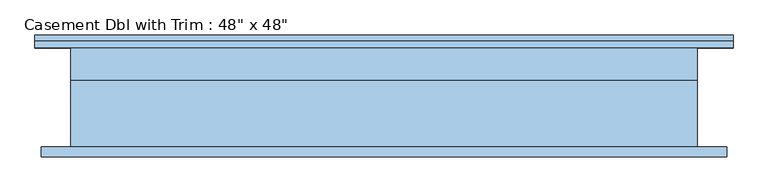
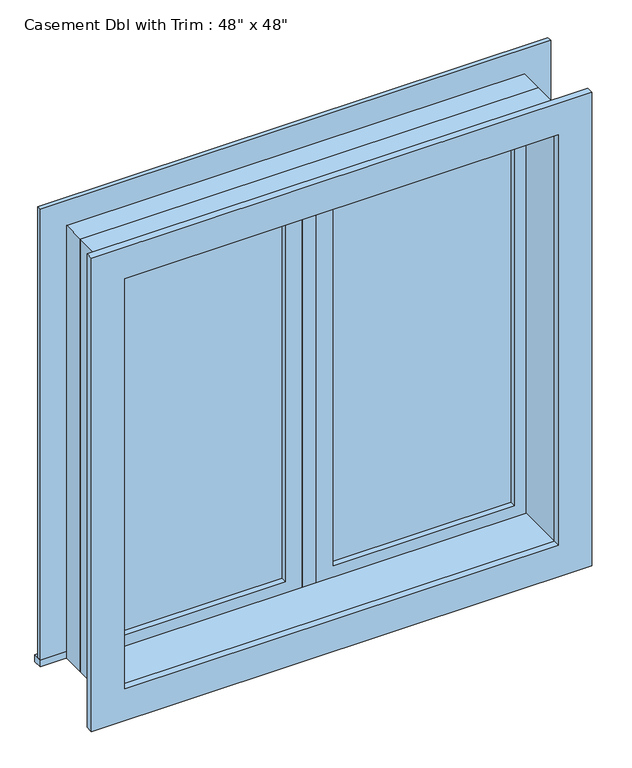
"""IFC4 building model written with IfcOpenShell, lengths in millimetres: window geometry."""

from ifc_helpers import new_model, si_unit, frame, origin, place, context, project, spatial, polyline, outline, extrude, source, transform, mapped, element, save


def window_d2c79e1c(model_context):
    return source(origin(), model_context, "Body", "SweptSolid", [
        extrude(outline(polyline([(63.5, 80.9625), (546.1, 80.9625), (546.1, 68.2625), (63.5, 68.2625), (63.5, 80.9625)])), frame((0.0, 0.0, 977.9), z_axis=(0.0, 0.0, 1.0), x_axis=(1.0, 0.0, 0.0)), (0.0, 0.0, 1.0), 1092.2),
        extrude(outline(polyline([(2114.55, 19.05), (933.45, 19.05), (933.45, 590.55), (2114.55, 590.55), (2114.55, 19.05)]), holes=[polyline([(2070.1, 63.5), (2070.1, 546.1), (977.9, 546.1), (977.9, 63.5), (2070.1, 63.5)])]), frame((0.0, 52.3875, 0.0), z_axis=(0.0, 1.0, 0.0), x_axis=(0.0, 0.0, 1.0)), (0.0, 0.0, 1.0), 44.45),
        extrude(outline(polyline([(19.05, 52.3875), (-19.05, 52.3875), (-19.05, 115.8875), (19.05, 115.8875), (19.05, 52.3875)])), frame((0.0, 0.0, 933.45), z_axis=(0.0, 0.0, 1.0), x_axis=(1.0, 0.0, 0.0)), (0.0, 0.0, 1.0), 1181.1),
        extrude(outline(polyline([(-679.45, 141.2875), (679.45, 141.2875), (679.45, 115.8875), (-679.45, 115.8875), (-679.45, 141.2875)])), frame((0.0, 0.0, 914.4), z_axis=(0.0, 0.0, 1.0), x_axis=(1.0, 0.0, 0.0)), (0.0, 0.0, 1.0), 19.05),
        extrude(outline(polyline([(2114.55, -590.55), (2114.55, 590.55), (933.45, 590.55), (933.45, 679.45), (2203.45, 679.45), (2203.45, -679.45), (933.45, -679.45), (933.45, -590.55), (2114.55, -590.55)])), frame((0.0, 115.8875, 0.0), z_axis=(0.0, 1.0, 0.0), x_axis=(0.0, 0.0, 1.0)), (0.0, 0.0, 1.0), 12.7),
        extrude(outline(polyline([(2190.75, 666.75), (2190.75, -666.75), (857.25, -666.75), (857.25, 666.75), (2190.75, 666.75)]), holes=[polyline([(2101.85, 577.85), (946.15, 577.85), (946.15, -577.85), (2101.85, -577.85), (2101.85, 577.85)])]), frame((0.0, -96.8375, 0.0), z_axis=(0.0, 1.0, 0.0), x_axis=(0.0, 0.0, 1.0)), (0.0, 0.0, 1.0), 19.05),
        extrude(outline(polyline([(-63.5, 68.2625), (-546.1, 68.2625), (-546.1, 80.9625), (-63.5, 80.9625), (-63.5, 68.2625)])), frame((0.0, 0.0, 977.9), z_axis=(0.0, 0.0, 1.0), x_axis=(1.0, 0.0, 0.0)), (0.0, 0.0, 1.0), 1092.2),
        extrude(outline(polyline([(2114.55, -590.55), (933.45, -590.55), (933.45, -19.05), (2114.55, -19.05), (2114.55, -590.55)]), holes=[polyline([(2070.1, -546.1), (2070.1, -63.5), (977.9, -63.5), (977.9, -546.1), (2070.1, -546.1)])]), frame((0.0, 52.3875, 0.0), z_axis=(0.0, 1.0, 0.0), x_axis=(0.0, 0.0, 1.0)), (0.0, 0.0, 1.0), 44.45),
        extrude(outline(polyline([(2133.6, -609.6), (914.4, -609.6), (914.4, 609.6), (2133.6, 609.6), (2133.6, -609.6)]), holes=[polyline([(2101.85, -577.85), (2101.85, 577.85), (946.15, 577.85), (946.15, -577.85), (2101.85, -577.85)])]), frame((0.0, -77.7875, 0.0), z_axis=(0.0, 1.0, 0.0), x_axis=(0.0, 0.0, 1.0)), (0.0, 0.0, 1.0), 130.175),
        extrude(outline(polyline([(2133.6, 609.6), (2133.6, -609.6), (914.4, -609.6), (914.4, 609.6), (2133.6, 609.6)]), holes=[polyline([(2114.55, 590.55), (933.45, 590.55), (933.45, -590.55), (2114.55, -590.55), (2114.55, 590.55)])]), frame((0.0, 52.3875, 0.0), z_axis=(0.0, 1.0, 0.0), x_axis=(0.0, 0.0, 1.0)), (0.0, 0.0, 1.0), 63.5),
    ])


if __name__ == "__main__":
    model = new_model("IFC4")
    model_context = context("Model", 3, world=origin())
    ifc_project = project(units=[si_unit("LENGTHUNIT", "METRE", prefix="MILLI")], contexts=[model_context])
    site = spatial("IfcSite", under=ifc_project)
    building = spatial("IfcBuilding", under=site)
    placement = place(None, origin())
    window_shape = window_d2c79e1c(model_context)
    element("IfcWindow", 1, ObjectType="Casement Dbl with Trim : 48\" x 48\"", at=placement, inside=building, context=model_context, shape_type="MappedRepresentation", body=[
        mapped(window_shape, transform((0.0, 0.0, 0.0), x_axis=(1.0, 0.0, 0.0), y_axis=(0.0, 1.0, 0.0), z_axis=(0.0, 0.0, 1.0))),
    ])
    save(model, "model.ifc")

# Revit data of these elements
# Type "Casement Dbl with Trim : 48\" x 48\""
#   Type Mark = "10"
#   Construction Type Id = "GSP4R"
#   Assembly Code = "B2020100"
#   Analytic Construction = "1/8 in Pilkington single glazing"
#   Visual Light Transmittance = 0.9
#   Solar Heat Gain Coefficient = 0.78
#   Heat Transfer Coefficient (U) = 0.6496 BTU/(h·ft²·°F)
#   Height = 4' - 0"
#   Default Sill Height = 3' - 0"
#   Trim Projection - Ext. = 0' - 0 1/2"
#   Trim Projection - Int. = 0' - 0 3/4"
#   Trim Width - Exterior = 0' - 3 1/2"
#   Trim Width - Interior = 0' - 3 1/2"
#   Width = 4' - 0"
#   Window Inset = 0' - 0 3/4"
#   Define Thermal Properties by = 1
#   Glass Pane Material = Glass
#   Sash Material = Sash
#   Trim Exterior Material = Trim
#   Trim Interior Material = Trim
#   Wall Closure = (empty or 0)
# Element 1 (IfcWindow, "Casement Dbl with Trim : 48\" x 48\"")
#   Materials on its faces: "Sash", "Trim", "Glass"
# Materials
#   "Glass": class "Glass", colour RGB 0 128 192, transparency 0.75, Description = "Soda Lime Glass", Cost = 0
#   "Sash": class "Wood", colour RGB 224 178 126, transparency 0
#   "Trim": class "Wood", colour RGB 224 178 126, transparency 0
